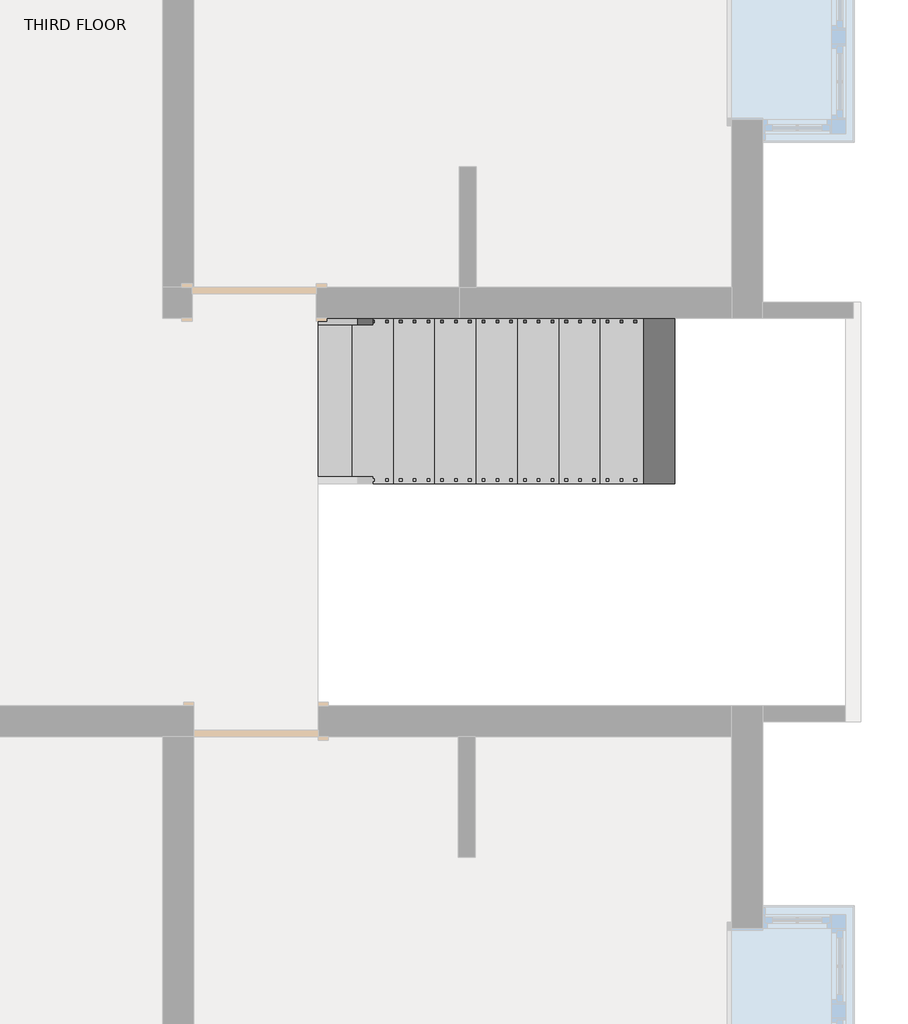
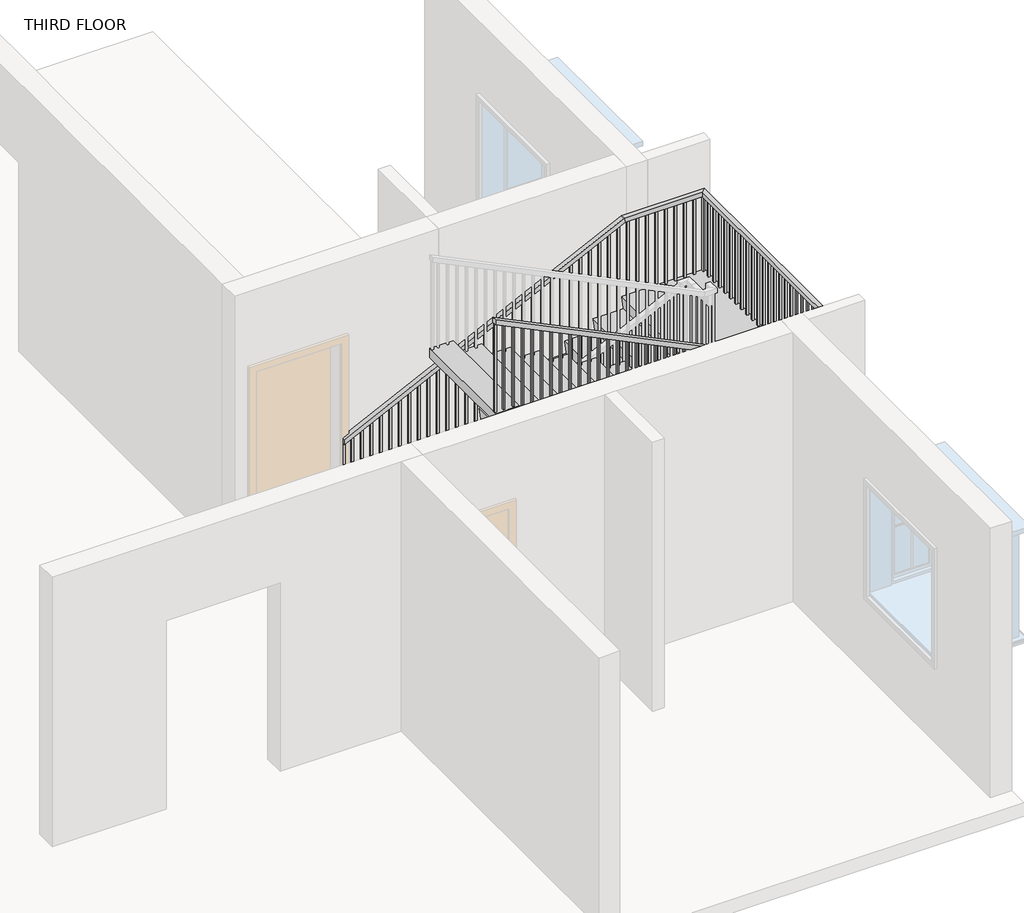
# One storey, part 3 of 4: 1 railing, 1 stair flight.
"""IFC4 building model written with IfcOpenShell, lengths in millimetres."""

from ifc_helpers import new_model, si_unit, frame, origin, place, context, project, spatial, polyline, outline, extrude, faceted_brep, element, save

model = new_model("IFC4")

# Units and contexts
model_context = context("Model", 3, world=origin())
ifc_project = project(units=[si_unit("LENGTHUNIT", "METRE", prefix="MILLI")], contexts=[model_context])

# Site, building, storey
site = spatial("IfcSite", under=ifc_project)
building = spatial("IfcBuilding", under=site)
storey = spatial("IfcBuildingStorey", under=building, Name="THIRD FLOOR", Elevation=9601.2)

# Railing
placement = place(None, origin())
element("IfcRailing", 1, ObjectType="Handrail - Rectangular", at=placement, inside=storey, context=model_context, shape_type="SolidModel", body=[
    faceted_brep([(3126.2584916, 220.733346, 10661.0727273), (3126.2584916, 220.733346, 10604.5956113), (3126.2584916, 169.933346, 10604.5956113), (3126.2584916, 169.933346, 10661.0727273), (6120.7829507, 220.733346, 12115.8), (6132.4691705, 220.733346, 12065.0), (6132.4691705, 169.933346, 12065.0), (6120.7829507, 169.933346, 12115.8), (7009.1350459, 220.733346, 12115.8), (7009.1350459, 220.733346, 12065.0), (6958.3350459, 169.933346, 12065.0), (6958.3350459, 169.933346, 12115.8), (7009.1350459, -2636.766654, 12115.8), (7009.1350459, -2636.766654, 12065.0), (6958.3350459, -2585.966654, 12065.0), (6958.3350459, -2585.966654, 12115.8), (6420.2353966, -2636.766654, 12115.8), (6408.5491768, -2636.766654, 12065.0), (6408.5491768, -2585.966654, 12065.0), (6420.2353966, -2585.966654, 12115.8), (3126.2584916, -2636.766654, 13716.0), (3126.2584916, -2585.966654, 13716.0), (3126.2584916, -2585.966654, 13659.522884), (3126.2584916, -2636.766654, 13659.522884)], [[[0, 1, 2, 3]], [[1, 0, 4, 5]], [[2, 1, 5, 6]], [[3, 2, 6, 7]], [[0, 3, 7, 4]], [[5, 4, 8, 9]], [[6, 5, 9, 10]], [[7, 6, 10, 11]], [[4, 7, 11, 8]], [[9, 8, 12, 13]], [[10, 9, 13, 14]], [[11, 10, 14, 15]], [[8, 11, 15, 12]], [[13, 12, 16, 17]], [[14, 13, 17, 18]], [[15, 14, 18, 19]], [[12, 15, 19, 16]], [[20, 21, 22, 23]], [[17, 16, 20, 23]], [[18, 17, 23, 22]], [[19, 18, 22, 21]], [[16, 19, 21, 20]]]),
    extrude(outline(polyline([(13616.4077556, 3215.0100459), (12656.1272727, 3215.0100459), (12656.1272727, 3234.0600459), (13607.1533465, 3234.0600459), (13616.4077556, 3215.0100459)])), frame((0.0, -2620.891654, 0.0), z_axis=(0.0, 1.0, 0.0), x_axis=(0.0, 0.0, 1.0)), (0.0, 0.0, 1.0), 19.05),
    extrude(outline(polyline([(13567.0509068, 3316.6100459), (12656.1272727, 3316.6100459), (12656.1272727, 3335.6600459), (13557.7964977, 3335.6600459), (13567.0509068, 3316.6100459)])), frame((0.0, -2620.891654, 0.0), z_axis=(0.0, 1.0, 0.0), x_axis=(0.0, 0.0, 1.0)), (0.0, 0.0, 1.0), 19.05),
    extrude(outline(polyline([(13517.694058, 3418.2100459), (12510.6545455, 3418.2100459), (12510.6545455, 3437.2600459), (13508.4396489, 3437.2600459), (13517.694058, 3418.2100459)])), frame((0.0, -2620.891654, 0.0), z_axis=(0.0, 1.0, 0.0), x_axis=(0.0, 0.0, 1.0)), (0.0, 0.0, 1.0), 19.05),
    extrude(outline(polyline([(13468.3372093, 3519.8100459), (12510.6545455, 3519.8100459), (12510.6545455, 3538.8600459), (13459.0828001, 3538.8600459), (13468.3372093, 3519.8100459)])), frame((0.0, -2620.891654, 0.0), z_axis=(0.0, 1.0, 0.0), x_axis=(0.0, 0.0, 1.0)), (0.0, 0.0, 1.0), 19.05),
    extrude(outline(polyline([(13418.9803605, 3621.4100459), (12510.6545455, 3621.4100459), (12510.6545455, 3640.4600459), (13409.7259513, 3640.4600459), (13418.9803605, 3621.4100459)])), frame((0.0, -2620.891654, 0.0), z_axis=(0.0, 1.0, 0.0), x_axis=(0.0, 0.0, 1.0)), (0.0, 0.0, 1.0), 19.05),
    extrude(outline(polyline([(13369.6235117, 3723.0100459), (12365.1818182, 3723.0100459), (12365.1818182, 3742.0600459), (13360.3691025, 3742.0600459), (13369.6235117, 3723.0100459)])), frame((0.0, -2620.891654, 0.0), z_axis=(0.0, 1.0, 0.0), x_axis=(0.0, 0.0, 1.0)), (0.0, 0.0, 1.0), 19.05),
    extrude(outline(polyline([(13320.2666629, 3824.6100459), (12365.1818182, 3824.6100459), (12365.1818182, 3843.6600459), (13311.0122538, 3843.6600459), (13320.2666629, 3824.6100459)])), frame((0.0, -2620.891654, 0.0), z_axis=(0.0, 1.0, 0.0), x_axis=(0.0, 0.0, 1.0)), (0.0, 0.0, 1.0), 19.05),
    extrude(outline(polyline([(13270.9098141, 3926.2100459), (12365.1818182, 3926.2100459), (12365.1818182, 3945.2600459), (13261.655405, 3945.2600459), (13270.9098141, 3926.2100459)])), frame((0.0, -2620.891654, 0.0), z_axis=(0.0, 1.0, 0.0), x_axis=(0.0, 0.0, 1.0)), (0.0, 0.0, 1.0), 19.05),
    extrude(outline(polyline([(13221.5529653, 4027.8100459), (12219.7090909, 4027.8100459), (12219.7090909, 4046.8600459), (13212.2985562, 4046.8600459), (13221.5529653, 4027.8100459)])), frame((0.0, -2620.891654, 0.0), z_axis=(0.0, 1.0, 0.0), x_axis=(0.0, 0.0, 1.0)), (0.0, 0.0, 1.0), 19.05),
    extrude(outline(polyline([(13172.1961165, 4129.4100459), (12219.7090909, 4129.4100459), (12219.7090909, 4148.4600459), (13162.9417074, 4148.4600459), (13172.1961165, 4129.4100459)])), frame((0.0, -2620.891654, 0.0), z_axis=(0.0, 1.0, 0.0), x_axis=(0.0, 0.0, 1.0)), (0.0, 0.0, 1.0), 19.05),
    extrude(outline(polyline([(13122.8392678, 4231.0100459), (12219.7090909, 4231.0100459), (12219.7090909, 4250.0600459), (13113.5848586, 4250.0600459), (13122.8392678, 4231.0100459)])), frame((0.0, -2620.891654, 0.0), z_axis=(0.0, 1.0, 0.0), x_axis=(0.0, 0.0, 1.0)), (0.0, 0.0, 1.0), 19.05),
    extrude(outline(polyline([(13073.482419, 4332.6100459), (12074.2363636, 4332.6100459), (12074.2363636, 4351.6600459), (13064.2280098, 4351.6600459), (13073.482419, 4332.6100459)])), frame((0.0, -2620.891654, 0.0), z_axis=(0.0, 1.0, 0.0), x_axis=(0.0, 0.0, 1.0)), (0.0, 0.0, 1.0), 19.05),
    extrude(outline(polyline([(13024.1255702, 4434.2100459), (12074.2363636, 4434.2100459), (12074.2363636, 4453.2600459), (13014.871161, 4453.2600459), (13024.1255702, 4434.2100459)])), frame((0.0, -2620.891654, 0.0), z_axis=(0.0, 1.0, 0.0), x_axis=(0.0, 0.0, 1.0)), (0.0, 0.0, 1.0), 19.05),
    extrude(outline(polyline([(12974.7687214, 4535.8100459), (12074.2363636, 4535.8100459), (12074.2363636, 4554.8600459), (12965.5143123, 4554.8600459), (12974.7687214, 4535.8100459)])), frame((0.0, -2620.891654, 0.0), z_axis=(0.0, 1.0, 0.0), x_axis=(0.0, 0.0, 1.0)), (0.0, 0.0, 1.0), 19.05),
    extrude(outline(polyline([(12925.4118726, 4637.4100459), (11928.7636364, 4637.4100459), (11928.7636364, 4656.4600459), (12916.1574635, 4656.4600459), (12925.4118726, 4637.4100459)])), frame((0.0, -2620.891654, 0.0), z_axis=(0.0, 1.0, 0.0), x_axis=(0.0, 0.0, 1.0)), (0.0, 0.0, 1.0), 19.05),
    extrude(outline(polyline([(12876.0550238, 4739.0100459), (11928.7636364, 4739.0100459), (11928.7636364, 4758.0600459), (12866.8006147, 4758.0600459), (12876.0550238, 4739.0100459)])), frame((0.0, -2620.891654, 0.0), z_axis=(0.0, 1.0, 0.0), x_axis=(0.0, 0.0, 1.0)), (0.0, 0.0, 1.0), 19.05),
    extrude(outline(polyline([(12826.6981751, 4840.6100459), (11928.7636364, 4840.6100459), (11928.7636364, 4859.6600459), (12817.4437659, 4859.6600459), (12826.6981751, 4840.6100459)])), frame((0.0, -2620.891654, 0.0), z_axis=(0.0, 1.0, 0.0), x_axis=(0.0, 0.0, 1.0)), (0.0, 0.0, 1.0), 19.05),
    extrude(outline(polyline([(12777.3413263, 4942.2100459), (11783.2909091, 4942.2100459), (11783.2909091, 4961.2600459), (12768.0869171, 4961.2600459), (12777.3413263, 4942.2100459)])), frame((0.0, -2620.891654, 0.0), z_axis=(0.0, 1.0, 0.0), x_axis=(0.0, 0.0, 1.0)), (0.0, 0.0, 1.0), 19.05),
    extrude(outline(polyline([(12727.9844775, 5043.8100459), (11783.2909091, 5043.8100459), (11783.2909091, 5062.8600459), (12718.7300683, 5062.8600459), (12727.9844775, 5043.8100459)])), frame((0.0, -2620.891654, 0.0), z_axis=(0.0, 1.0, 0.0), x_axis=(0.0, 0.0, 1.0)), (0.0, 0.0, 1.0), 19.05),
    extrude(outline(polyline([(12678.6276287, 5145.4100459), (11783.2909091, 5145.4100459), (11783.2909091, 5164.4600459), (12669.3732196, 5164.4600459), (12678.6276287, 5145.4100459)])), frame((0.0, -2620.891654, 0.0), z_axis=(0.0, 1.0, 0.0), x_axis=(0.0, 0.0, 1.0)), (0.0, 0.0, 1.0), 19.05),
    extrude(outline(polyline([(12629.2707799, 5247.0100459), (11637.8181818, 5247.0100459), (11637.8181818, 5266.0600459), (12620.0163708, 5266.0600459), (12629.2707799, 5247.0100459)])), frame((0.0, -2620.891654, 0.0), z_axis=(0.0, 1.0, 0.0), x_axis=(0.0, 0.0, 1.0)), (0.0, 0.0, 1.0), 19.05),
    extrude(outline(polyline([(12579.9139311, 5348.6100459), (11637.8181818, 5348.6100459), (11637.8181818, 5367.6600459), (12570.659522, 5367.6600459), (12579.9139311, 5348.6100459)])), frame((0.0, -2620.891654, 0.0), z_axis=(0.0, 1.0, 0.0), x_axis=(0.0, 0.0, 1.0)), (0.0, 0.0, 1.0), 19.05),
    extrude(outline(polyline([(12530.5570823, 5450.2100459), (11637.8181818, 5450.2100459), (11637.8181818, 5469.2600459), (12521.3026732, 5469.2600459), (12530.5570823, 5450.2100459)])), frame((0.0, -2620.891654, 0.0), z_axis=(0.0, 1.0, 0.0), x_axis=(0.0, 0.0, 1.0)), (0.0, 0.0, 1.0), 19.05),
    extrude(outline(polyline([(12481.2002336, 5551.8100459), (11492.3454545, 5551.8100459), (11492.3454545, 5570.8600459), (12471.9458244, 5570.8600459), (12481.2002336, 5551.8100459)])), frame((0.0, -2620.891654, 0.0), z_axis=(0.0, 1.0, 0.0), x_axis=(0.0, 0.0, 1.0)), (0.0, 0.0, 1.0), 19.05),
    extrude(outline(polyline([(12431.8433848, 5653.4100459), (11492.3454545, 5653.4100459), (11492.3454545, 5672.4600459), (12422.5889756, 5672.4600459), (12431.8433848, 5653.4100459)])), frame((0.0, -2620.891654, 0.0), z_axis=(0.0, 1.0, 0.0), x_axis=(0.0, 0.0, 1.0)), (0.0, 0.0, 1.0), 19.05),
    extrude(outline(polyline([(12382.486536, 5755.0100459), (11492.3454545, 5755.0100459), (11492.3454545, 5774.0600459), (12373.2321268, 5774.0600459), (12382.486536, 5755.0100459)])), frame((0.0, -2620.891654, 0.0), z_axis=(0.0, 1.0, 0.0), x_axis=(0.0, 0.0, 1.0)), (0.0, 0.0, 1.0), 19.05),
    extrude(outline(polyline([(12333.1296872, 5856.6100459), (11346.8727273, 5856.6100459), (11346.8727273, 5875.6600459), (12323.8752781, 5875.6600459), (12333.1296872, 5856.6100459)])), frame((0.0, -2620.891654, 0.0), z_axis=(0.0, 1.0, 0.0), x_axis=(0.0, 0.0, 1.0)), (0.0, 0.0, 1.0), 19.05),
    extrude(outline(polyline([(12283.7728384, 5958.2100459), (11346.8727273, 5958.2100459), (11346.8727273, 5977.2600459), (12274.5184293, 5977.2600459), (12283.7728384, 5958.2100459)])), frame((0.0, -2620.891654, 0.0), z_axis=(0.0, 1.0, 0.0), x_axis=(0.0, 0.0, 1.0)), (0.0, 0.0, 1.0), 19.05),
    extrude(outline(polyline([(12234.4159896, 6059.8100459), (11346.8727273, 6059.8100459), (11346.8727273, 6078.8600459), (12225.1615805, 6078.8600459), (12234.4159896, 6059.8100459)])), frame((0.0, -2620.891654, 0.0), z_axis=(0.0, 1.0, 0.0), x_axis=(0.0, 0.0, 1.0)), (0.0, 0.0, 1.0), 19.05),
    extrude(outline(polyline([(12185.0591409, 6161.4100459), (11201.4, 6161.4100459), (11201.4, 6180.4600459), (12175.8047317, 6180.4600459), (12185.0591409, 6161.4100459)])), frame((0.0, -2620.891654, 0.0), z_axis=(0.0, 1.0, 0.0), x_axis=(0.0, 0.0, 1.0)), (0.0, 0.0, 1.0), 19.05),
    extrude(outline(polyline([(12135.7022921, 6263.0100459), (11201.4, 6263.0100459), (11201.4, 6282.0600459), (12126.4478829, 6282.0600459), (12135.7022921, 6263.0100459)])), frame((0.0, -2620.891654, 0.0), z_axis=(0.0, 1.0, 0.0), x_axis=(0.0, 0.0, 1.0)), (0.0, 0.0, 1.0), 19.05),
    extrude(outline(polyline([(12086.3454433, 6364.6100459), (11201.4, 6364.6100459), (11201.4, 6383.6600459), (12077.0910341, 6383.6600459), (12086.3454433, 6364.6100459)])), frame((0.0, -2620.891654, 0.0), z_axis=(0.0, 1.0, 0.0), x_axis=(0.0, 0.0, 1.0)), (0.0, 0.0, 1.0), 19.05),
    extrude(outline(polyline([(6485.2600459, -2620.891654), (6466.2100459, -2620.891654), (6466.2100459, -2601.841654), (6485.2600459, -2601.841654), (6485.2600459, -2620.891654)])), frame((0.0, 0.0, 11201.4), z_axis=(0.0, 0.0, 1.0), x_axis=(1.0, 0.0, 0.0)), (0.0, 0.0, 1.0), 863.6),
    extrude(outline(polyline([(6586.8600459, -2620.891654), (6567.8100459, -2620.891654), (6567.8100459, -2601.841654), (6586.8600459, -2601.841654), (6586.8600459, -2620.891654)])), frame((0.0, 0.0, 11201.4), z_axis=(0.0, 0.0, 1.0), x_axis=(1.0, 0.0, 0.0)), (0.0, 0.0, 1.0), 863.6),
    extrude(outline(polyline([(6688.4600459, -2620.891654), (6669.4100459, -2620.891654), (6669.4100459, -2601.841654), (6688.4600459, -2601.841654), (6688.4600459, -2620.891654)])), frame((0.0, 0.0, 11201.4), z_axis=(0.0, 0.0, 1.0), x_axis=(1.0, 0.0, 0.0)), (0.0, 0.0, 1.0), 863.6),
    extrude(outline(polyline([(6790.0600459, -2620.891654), (6771.0100459, -2620.891654), (6771.0100459, -2601.841654), (6790.0600459, -2601.841654), (6790.0600459, -2620.891654)])), frame((0.0, 0.0, 11201.4), z_axis=(0.0, 0.0, 1.0), x_axis=(1.0, 0.0, 0.0)), (0.0, 0.0, 1.0), 863.6),
    extrude(outline(polyline([(6891.6600459, -2620.891654), (6872.6100459, -2620.891654), (6872.6100459, -2601.841654), (6891.6600459, -2601.841654), (6891.6600459, -2620.891654)])), frame((0.0, 0.0, 11201.4), z_axis=(0.0, 0.0, 1.0), x_axis=(1.0, 0.0, 0.0)), (0.0, 0.0, 1.0), 863.6),
    extrude(outline(polyline([(6993.2600459, -2538.341654), (6993.2600459, -2557.391654), (6974.2100459, -2557.391654), (6974.2100459, -2538.341654), (6993.2600459, -2538.341654)])), frame((0.0, 0.0, 11201.4), z_axis=(0.0, 0.0, 1.0), x_axis=(1.0, 0.0, 0.0)), (0.0, 0.0, 1.0), 863.6),
    extrude(outline(polyline([(6993.2600459, -2436.741654), (6993.2600459, -2455.791654), (6974.2100459, -2455.791654), (6974.2100459, -2436.741654), (6993.2600459, -2436.741654)])), frame((0.0, 0.0, 11201.4), z_axis=(0.0, 0.0, 1.0), x_axis=(1.0, 0.0, 0.0)), (0.0, 0.0, 1.0), 863.6),
    extrude(outline(polyline([(6993.2600459, -2335.141654), (6993.2600459, -2354.191654), (6974.2100459, -2354.191654), (6974.2100459, -2335.141654), (6993.2600459, -2335.141654)])), frame((0.0, 0.0, 11201.4), z_axis=(0.0, 0.0, 1.0), x_axis=(1.0, 0.0, 0.0)), (0.0, 0.0, 1.0), 863.6),
    extrude(outline(polyline([(6993.2600459, -2233.541654), (6993.2600459, -2252.591654), (6974.2100459, -2252.591654), (6974.2100459, -2233.541654), (6993.2600459, -2233.541654)])), frame((0.0, 0.0, 11201.4), z_axis=(0.0, 0.0, 1.0), x_axis=(1.0, 0.0, 0.0)), (0.0, 0.0, 1.0), 863.6),
    extrude(outline(polyline([(6993.2600459, -2131.941654), (6993.2600459, -2150.991654), (6974.2100459, -2150.991654), (6974.2100459, -2131.941654), (6993.2600459, -2131.941654)])), frame((0.0, 0.0, 11201.4), z_axis=(0.0, 0.0, 1.0), x_axis=(1.0, 0.0, 0.0)), (0.0, 0.0, 1.0), 863.6),
    extrude(outline(polyline([(6993.2600459, -2030.341654), (6993.2600459, -2049.391654), (6974.2100459, -2049.391654), (6974.2100459, -2030.341654), (6993.2600459, -2030.341654)])), frame((0.0, 0.0, 11201.4), z_axis=(0.0, 0.0, 1.0), x_axis=(1.0, 0.0, 0.0)), (0.0, 0.0, 1.0), 863.6),
    extrude(outline(polyline([(6993.2600459, -1928.741654), (6993.2600459, -1947.791654), (6974.2100459, -1947.791654), (6974.2100459, -1928.741654), (6993.2600459, -1928.741654)])), frame((0.0, 0.0, 11201.4), z_axis=(0.0, 0.0, 1.0), x_axis=(1.0, 0.0, 0.0)), (0.0, 0.0, 1.0), 863.6),
    extrude(outline(polyline([(6993.2600459, -1827.141654), (6993.2600459, -1846.191654), (6974.2100459, -1846.191654), (6974.2100459, -1827.141654), (6993.2600459, -1827.141654)])), frame((0.0, 0.0, 11201.4), z_axis=(0.0, 0.0, 1.0), x_axis=(1.0, 0.0, 0.0)), (0.0, 0.0, 1.0), 863.6),
    extrude(outline(polyline([(6993.2600459, -1725.541654), (6993.2600459, -1744.591654), (6974.2100459, -1744.591654), (6974.2100459, -1725.541654), (6993.2600459, -1725.541654)])), frame((0.0, 0.0, 11201.4), z_axis=(0.0, 0.0, 1.0), x_axis=(1.0, 0.0, 0.0)), (0.0, 0.0, 1.0), 863.6),
    extrude(outline(polyline([(6993.2600459, -1623.941654), (6993.2600459, -1642.991654), (6974.2100459, -1642.991654), (6974.2100459, -1623.941654), (6993.2600459, -1623.941654)])), frame((0.0, 0.0, 11201.4), z_axis=(0.0, 0.0, 1.0), x_axis=(1.0, 0.0, 0.0)), (0.0, 0.0, 1.0), 863.6),
    extrude(outline(polyline([(6993.2600459, -1522.341654), (6993.2600459, -1541.391654), (6974.2100459, -1541.391654), (6974.2100459, -1522.341654), (6993.2600459, -1522.341654)])), frame((0.0, 0.0, 11201.4), z_axis=(0.0, 0.0, 1.0), x_axis=(1.0, 0.0, 0.0)), (0.0, 0.0, 1.0), 863.6),
    extrude(outline(polyline([(6993.2600459, -1420.741654), (6993.2600459, -1439.791654), (6974.2100459, -1439.791654), (6974.2100459, -1420.741654), (6993.2600459, -1420.741654)])), frame((0.0, 0.0, 11201.4), z_axis=(0.0, 0.0, 1.0), x_axis=(1.0, 0.0, 0.0)), (0.0, 0.0, 1.0), 863.6),
    extrude(outline(polyline([(6993.2600459, -1319.141654), (6993.2600459, -1338.191654), (6974.2100459, -1338.191654), (6974.2100459, -1319.141654), (6993.2600459, -1319.141654)])), frame((0.0, 0.0, 11201.4), z_axis=(0.0, 0.0, 1.0), x_axis=(1.0, 0.0, 0.0)), (0.0, 0.0, 1.0), 863.6),
    extrude(outline(polyline([(6993.2600459, -1217.541654), (6993.2600459, -1236.591654), (6974.2100459, -1236.591654), (6974.2100459, -1217.541654), (6993.2600459, -1217.541654)])), frame((0.0, 0.0, 11201.4), z_axis=(0.0, 0.0, 1.0), x_axis=(1.0, 0.0, 0.0)), (0.0, 0.0, 1.0), 863.6),
    extrude(outline(polyline([(6993.2600459, -1115.941654), (6993.2600459, -1134.991654), (6974.2100459, -1134.991654), (6974.2100459, -1115.941654), (6993.2600459, -1115.941654)])), frame((0.0, 0.0, 11201.4), z_axis=(0.0, 0.0, 1.0), x_axis=(1.0, 0.0, 0.0)), (0.0, 0.0, 1.0), 863.6),
    extrude(outline(polyline([(6993.2600459, -1014.341654), (6993.2600459, -1033.391654), (6974.2100459, -1033.391654), (6974.2100459, -1014.341654), (6993.2600459, -1014.341654)])), frame((0.0, 0.0, 11201.4), z_axis=(0.0, 0.0, 1.0), x_axis=(1.0, 0.0, 0.0)), (0.0, 0.0, 1.0), 863.6),
    extrude(outline(polyline([(6993.2600459, -912.741654), (6993.2600459, -931.791654), (6974.2100459, -931.791654), (6974.2100459, -912.741654), (6993.2600459, -912.741654)])), frame((0.0, 0.0, 11201.4), z_axis=(0.0, 0.0, 1.0), x_axis=(1.0, 0.0, 0.0)), (0.0, 0.0, 1.0), 863.6),
    extrude(outline(polyline([(6993.2600459, -811.141654), (6993.2600459, -830.191654), (6974.2100459, -830.191654), (6974.2100459, -811.141654), (6993.2600459, -811.141654)])), frame((0.0, 0.0, 11201.4), z_axis=(0.0, 0.0, 1.0), x_axis=(1.0, 0.0, 0.0)), (0.0, 0.0, 1.0), 863.6),
    extrude(outline(polyline([(6993.2600459, -709.541654), (6993.2600459, -728.591654), (6974.2100459, -728.591654), (6974.2100459, -709.541654), (6993.2600459, -709.541654)])), frame((0.0, 0.0, 11201.4), z_axis=(0.0, 0.0, 1.0), x_axis=(1.0, 0.0, 0.0)), (0.0, 0.0, 1.0), 863.6),
    extrude(outline(polyline([(6993.2600459, -607.941654), (6993.2600459, -626.991654), (6974.2100459, -626.991654), (6974.2100459, -607.941654), (6993.2600459, -607.941654)])), frame((0.0, 0.0, 11201.4), z_axis=(0.0, 0.0, 1.0), x_axis=(1.0, 0.0, 0.0)), (0.0, 0.0, 1.0), 863.6),
    extrude(outline(polyline([(6993.2600459, -506.341654), (6993.2600459, -525.391654), (6974.2100459, -525.391654), (6974.2100459, -506.341654), (6993.2600459, -506.341654)])), frame((0.0, 0.0, 11201.4), z_axis=(0.0, 0.0, 1.0), x_axis=(1.0, 0.0, 0.0)), (0.0, 0.0, 1.0), 863.6),
    extrude(outline(polyline([(6993.2600459, -404.741654), (6993.2600459, -423.791654), (6974.2100459, -423.791654), (6974.2100459, -404.741654), (6993.2600459, -404.741654)])), frame((0.0, 0.0, 11201.4), z_axis=(0.0, 0.0, 1.0), x_axis=(1.0, 0.0, 0.0)), (0.0, 0.0, 1.0), 863.6),
    extrude(outline(polyline([(6993.2600459, -303.141654), (6993.2600459, -322.191654), (6974.2100459, -322.191654), (6974.2100459, -303.141654), (6993.2600459, -303.141654)])), frame((0.0, 0.0, 11201.4), z_axis=(0.0, 0.0, 1.0), x_axis=(1.0, 0.0, 0.0)), (0.0, 0.0, 1.0), 863.6),
    extrude(outline(polyline([(6993.2600459, -201.541654), (6993.2600459, -220.591654), (6974.2100459, -220.591654), (6974.2100459, -201.541654), (6993.2600459, -201.541654)])), frame((0.0, 0.0, 11201.4), z_axis=(0.0, 0.0, 1.0), x_axis=(1.0, 0.0, 0.0)), (0.0, 0.0, 1.0), 863.6),
    extrude(outline(polyline([(6993.2600459, -99.941654), (6993.2600459, -118.991654), (6974.2100459, -118.991654), (6974.2100459, -99.941654), (6993.2600459, -99.941654)])), frame((0.0, 0.0, 11201.4), z_axis=(0.0, 0.0, 1.0), x_axis=(1.0, 0.0, 0.0)), (0.0, 0.0, 1.0), 863.6),
    extrude(outline(polyline([(6993.2600459, 1.658346), (6993.2600459, -17.391654), (6974.2100459, -17.391654), (6974.2100459, 1.658346), (6993.2600459, 1.658346)])), frame((0.0, 0.0, 11201.4), z_axis=(0.0, 0.0, 1.0), x_axis=(1.0, 0.0, 0.0)), (0.0, 0.0, 1.0), 863.6),
    extrude(outline(polyline([(6993.2600459, 103.258346), (6993.2600459, 84.208346), (6974.2100459, 84.208346), (6974.2100459, 103.258346), (6993.2600459, 103.258346)])), frame((0.0, 0.0, 11201.4), z_axis=(0.0, 0.0, 1.0), x_axis=(1.0, 0.0, 0.0)), (0.0, 0.0, 1.0), 863.6),
    extrude(outline(polyline([(6875.9334916, 204.858346), (6894.9834916, 204.858346), (6894.9834916, 185.808346), (6875.9334916, 185.808346), (6875.9334916, 204.858346)])), frame((0.0, 0.0, 11201.4), z_axis=(0.0, 0.0, 1.0), x_axis=(1.0, 0.0, 0.0)), (0.0, 0.0, 1.0), 863.6),
    extrude(outline(polyline([(6774.3334916, 204.858346), (6793.3834916, 204.858346), (6793.3834916, 185.808346), (6774.3334916, 185.808346), (6774.3334916, 204.858346)])), frame((0.0, 0.0, 11201.4), z_axis=(0.0, 0.0, 1.0), x_axis=(1.0, 0.0, 0.0)), (0.0, 0.0, 1.0), 863.6),
    extrude(outline(polyline([(6672.7334916, 204.858346), (6691.7834916, 204.858346), (6691.7834916, 185.808346), (6672.7334916, 185.808346), (6672.7334916, 204.858346)])), frame((0.0, 0.0, 11201.4), z_axis=(0.0, 0.0, 1.0), x_axis=(1.0, 0.0, 0.0)), (0.0, 0.0, 1.0), 863.6),
    extrude(outline(polyline([(6571.1334916, 204.858346), (6590.1834916, 204.858346), (6590.1834916, 185.808346), (6571.1334916, 185.808346), (6571.1334916, 204.858346)])), frame((0.0, 0.0, 11201.4), z_axis=(0.0, 0.0, 1.0), x_axis=(1.0, 0.0, 0.0)), (0.0, 0.0, 1.0), 863.6),
    extrude(outline(polyline([(6469.5334916, 204.858346), (6488.5834916, 204.858346), (6488.5834916, 185.808346), (6469.5334916, 185.808346), (6469.5334916, 204.858346)])), frame((0.0, 0.0, 11201.4), z_axis=(0.0, 0.0, 1.0), x_axis=(1.0, 0.0, 0.0)), (0.0, 0.0, 1.0), 863.6),
    extrude(outline(polyline([(6367.9334916, 204.858346), (6386.9834916, 204.858346), (6386.9834916, 185.808346), (6367.9334916, 185.808346), (6367.9334916, 204.858346)])), frame((0.0, 0.0, 11201.4), z_axis=(0.0, 0.0, 1.0), x_axis=(1.0, 0.0, 0.0)), (0.0, 0.0, 1.0), 863.6),
    extrude(outline(polyline([(6266.3334916, 204.858346), (6285.3834916, 204.858346), (6285.3834916, 185.808346), (6266.3334916, 185.808346), (6266.3334916, 204.858346)])), frame((0.0, 0.0, 11201.4), z_axis=(0.0, 0.0, 1.0), x_axis=(1.0, 0.0, 0.0)), (0.0, 0.0, 1.0), 863.6),
    extrude(outline(polyline([(6164.7334916, 204.858346), (6183.7834916, 204.858346), (6183.7834916, 185.808346), (6164.7334916, 185.808346), (6164.7334916, 204.858346)])), frame((0.0, 0.0, 11201.4), z_axis=(0.0, 0.0, 1.0), x_axis=(1.0, 0.0, 0.0)), (0.0, 0.0, 1.0), 863.6),
    extrude(outline(polyline([(12031.3170215, 6063.1334916), (11055.9272727, 6063.1334916), (11055.9272727, 6082.1834916), (12040.5714306, 6082.1834916), (12031.3170215, 6063.1334916)])), frame((0.0, 185.808346, 0.0), z_axis=(0.0, 1.0, 0.0), x_axis=(0.0, 0.0, 1.0)), (0.0, 0.0, 1.0), 19.05),
    extrude(outline(polyline([(11981.9601727, 5961.5334916), (11055.9272727, 5961.5334916), (11055.9272727, 5980.5834916), (11991.2145818, 5980.5834916), (11981.9601727, 5961.5334916)])), frame((0.0, 185.808346, 0.0), z_axis=(0.0, 1.0, 0.0), x_axis=(0.0, 0.0, 1.0)), (0.0, 0.0, 1.0), 19.05),
    extrude(outline(polyline([(11932.6033239, 5859.9334916), (11055.9272727, 5859.9334916), (11055.9272727, 5878.9834916), (11941.857733, 5878.9834916), (11932.6033239, 5859.9334916)])), frame((0.0, 185.808346, 0.0), z_axis=(0.0, 1.0, 0.0), x_axis=(0.0, 0.0, 1.0)), (0.0, 0.0, 1.0), 19.05),
    extrude(outline(polyline([(11883.2464751, 5758.3334916), (10910.4545455, 5758.3334916), (10910.4545455, 5777.3834916), (11892.5008843, 5777.3834916), (11883.2464751, 5758.3334916)])), frame((0.0, 185.808346, 0.0), z_axis=(0.0, 1.0, 0.0), x_axis=(0.0, 0.0, 1.0)), (0.0, 0.0, 1.0), 19.05),
    extrude(outline(polyline([(11833.8896263, 5656.7334916), (10910.4545455, 5656.7334916), (10910.4545455, 5675.7834916), (11843.1440355, 5675.7834916), (11833.8896263, 5656.7334916)])), frame((0.0, 185.808346, 0.0), z_axis=(0.0, 1.0, 0.0), x_axis=(0.0, 0.0, 1.0)), (0.0, 0.0, 1.0), 19.05),
    extrude(outline(polyline([(11784.5327775, 5555.1334916), (10910.4545455, 5555.1334916), (10910.4545455, 5574.1834916), (11793.7871867, 5574.1834916), (11784.5327775, 5555.1334916)])), frame((0.0, 185.808346, 0.0), z_axis=(0.0, 1.0, 0.0), x_axis=(0.0, 0.0, 1.0)), (0.0, 0.0, 1.0), 19.05),
    extrude(outline(polyline([(11735.1759288, 5453.5334916), (10764.9818182, 5453.5334916), (10764.9818182, 5472.5834916), (11744.4303379, 5472.5834916), (11735.1759288, 5453.5334916)])), frame((0.0, 185.808346, 0.0), z_axis=(0.0, 1.0, 0.0), x_axis=(0.0, 0.0, 1.0)), (0.0, 0.0, 1.0), 19.05),
    extrude(outline(polyline([(11685.81908, 5351.9334916), (10764.9818182, 5351.9334916), (10764.9818182, 5370.9834916), (11695.0734891, 5370.9834916), (11685.81908, 5351.9334916)])), frame((0.0, 185.808346, 0.0), z_axis=(0.0, 1.0, 0.0), x_axis=(0.0, 0.0, 1.0)), (0.0, 0.0, 1.0), 19.05),
    extrude(outline(polyline([(11636.4622312, 5250.3334916), (10764.9818182, 5250.3334916), (10764.9818182, 5269.3834916), (11645.7166403, 5269.3834916), (11636.4622312, 5250.3334916)])), frame((0.0, 185.808346, 0.0), z_axis=(0.0, 1.0, 0.0), x_axis=(0.0, 0.0, 1.0)), (0.0, 0.0, 1.0), 19.05),
    extrude(outline(polyline([(11587.1053824, 5148.7334916), (10619.5090909, 5148.7334916), (10619.5090909, 5167.7834916), (11596.3597915, 5167.7834916), (11587.1053824, 5148.7334916)])), frame((0.0, 185.808346, 0.0), z_axis=(0.0, 1.0, 0.0), x_axis=(0.0, 0.0, 1.0)), (0.0, 0.0, 1.0), 19.05),
    extrude(outline(polyline([(11537.7485336, 5047.1334916), (10619.5090909, 5047.1334916), (10619.5090909, 5066.1834916), (11547.0029428, 5066.1834916), (11537.7485336, 5047.1334916)])), frame((0.0, 185.808346, 0.0), z_axis=(0.0, 1.0, 0.0), x_axis=(0.0, 0.0, 1.0)), (0.0, 0.0, 1.0), 19.05),
    extrude(outline(polyline([(11488.3916848, 4945.5334916), (10619.5090909, 4945.5334916), (10619.5090909, 4964.5834916), (11497.646094, 4964.5834916), (11488.3916848, 4945.5334916)])), frame((0.0, 185.808346, 0.0), z_axis=(0.0, 1.0, 0.0), x_axis=(0.0, 0.0, 1.0)), (0.0, 0.0, 1.0), 19.05),
    extrude(outline(polyline([(11439.034836, 4843.9334916), (10474.0363636, 4843.9334916), (10474.0363636, 4862.9834916), (11448.2892452, 4862.9834916), (11439.034836, 4843.9334916)])), frame((0.0, 185.808346, 0.0), z_axis=(0.0, 1.0, 0.0), x_axis=(0.0, 0.0, 1.0)), (0.0, 0.0, 1.0), 19.05),
    extrude(outline(polyline([(11389.6779873, 4742.3334916), (10474.0363636, 4742.3334916), (10474.0363636, 4761.3834916), (11398.9323964, 4761.3834916), (11389.6779873, 4742.3334916)])), frame((0.0, 185.808346, 0.0), z_axis=(0.0, 1.0, 0.0), x_axis=(0.0, 0.0, 1.0)), (0.0, 0.0, 1.0), 19.05),
    extrude(outline(polyline([(11340.3211385, 4640.7334916), (10474.0363636, 4640.7334916), (10474.0363636, 4659.7834916), (11349.5755476, 4659.7834916), (11340.3211385, 4640.7334916)])), frame((0.0, 185.808346, 0.0), z_axis=(0.0, 1.0, 0.0), x_axis=(0.0, 0.0, 1.0)), (0.0, 0.0, 1.0), 19.05),
    extrude(outline(polyline([(11290.9642897, 4539.1334916), (10328.5636364, 4539.1334916), (10328.5636364, 4558.1834916), (11300.2186988, 4558.1834916), (11290.9642897, 4539.1334916)])), frame((0.0, 185.808346, 0.0), z_axis=(0.0, 1.0, 0.0), x_axis=(0.0, 0.0, 1.0)), (0.0, 0.0, 1.0), 19.05),
    extrude(outline(polyline([(11241.6074409, 4437.5334916), (10328.5636364, 4437.5334916), (10328.5636364, 4456.5834916), (11250.8618501, 4456.5834916), (11241.6074409, 4437.5334916)])), frame((0.0, 185.808346, 0.0), z_axis=(0.0, 1.0, 0.0), x_axis=(0.0, 0.0, 1.0)), (0.0, 0.0, 1.0), 19.05),
    extrude(outline(polyline([(11192.2505921, 4335.9334916), (10328.5636364, 4335.9334916), (10328.5636364, 4354.9834916), (11201.5050013, 4354.9834916), (11192.2505921, 4335.9334916)])), frame((0.0, 185.808346, 0.0), z_axis=(0.0, 1.0, 0.0), x_axis=(0.0, 0.0, 1.0)), (0.0, 0.0, 1.0), 19.05),
    extrude(outline(polyline([(11142.8937433, 4234.3334916), (10183.0909091, 4234.3334916), (10183.0909091, 4253.3834916), (11152.1481525, 4253.3834916), (11142.8937433, 4234.3334916)])), frame((0.0, 185.808346, 0.0), z_axis=(0.0, 1.0, 0.0), x_axis=(0.0, 0.0, 1.0)), (0.0, 0.0, 1.0), 19.05),
    extrude(outline(polyline([(11093.5368946, 4132.7334916), (10183.0909091, 4132.7334916), (10183.0909091, 4151.7834916), (11102.7913037, 4151.7834916), (11093.5368946, 4132.7334916)])), frame((0.0, 185.808346, 0.0), z_axis=(0.0, 1.0, 0.0), x_axis=(0.0, 0.0, 1.0)), (0.0, 0.0, 1.0), 19.05),
    extrude(outline(polyline([(11044.1800458, 4031.1334916), (10183.0909091, 4031.1334916), (10183.0909091, 4050.1834916), (11053.4344549, 4050.1834916), (11044.1800458, 4031.1334916)])), frame((0.0, 185.808346, 0.0), z_axis=(0.0, 1.0, 0.0), x_axis=(0.0, 0.0, 1.0)), (0.0, 0.0, 1.0), 19.05),
    extrude(outline(polyline([(10994.823197, 3929.5334916), (10037.6181818, 3929.5334916), (10037.6181818, 3948.5834916), (11004.0776061, 3948.5834916), (10994.823197, 3929.5334916)])), frame((0.0, 185.808346, 0.0), z_axis=(0.0, 1.0, 0.0), x_axis=(0.0, 0.0, 1.0)), (0.0, 0.0, 1.0), 19.05),
    extrude(outline(polyline([(10945.4663482, 3827.9334916), (10037.6181818, 3827.9334916), (10037.6181818, 3846.9834916), (10954.7207573, 3846.9834916), (10945.4663482, 3827.9334916)])), frame((0.0, 185.808346, 0.0), z_axis=(0.0, 1.0, 0.0), x_axis=(0.0, 0.0, 1.0)), (0.0, 0.0, 1.0), 19.05),
    extrude(outline(polyline([(10896.1094994, 3726.3334916), (10037.6181818, 3726.3334916), (10037.6181818, 3745.3834916), (10905.3639086, 3745.3834916), (10896.1094994, 3726.3334916)])), frame((0.0, 185.808346, 0.0), z_axis=(0.0, 1.0, 0.0), x_axis=(0.0, 0.0, 1.0)), (0.0, 0.0, 1.0), 19.05),
    extrude(outline(polyline([(10846.7526506, 3624.7334916), (9892.1454545, 3624.7334916), (9892.1454545, 3643.7834916), (10856.0070598, 3643.7834916), (10846.7526506, 3624.7334916)])), frame((0.0, 185.808346, 0.0), z_axis=(0.0, 1.0, 0.0), x_axis=(0.0, 0.0, 1.0)), (0.0, 0.0, 1.0), 19.05),
    extrude(outline(polyline([(10797.3958018, 3523.1334916), (9892.1454545, 3523.1334916), (9892.1454545, 3542.1834916), (10806.650211, 3542.1834916), (10797.3958018, 3523.1334916)])), frame((0.0, 185.808346, 0.0), z_axis=(0.0, 1.0, 0.0), x_axis=(0.0, 0.0, 1.0)), (0.0, 0.0, 1.0), 19.05),
    extrude(outline(polyline([(10748.0389531, 3421.5334916), (9892.1454545, 3421.5334916), (9892.1454545, 3440.5834916), (10757.2933622, 3440.5834916), (10748.0389531, 3421.5334916)])), frame((0.0, 185.808346, 0.0), z_axis=(0.0, 1.0, 0.0), x_axis=(0.0, 0.0, 1.0)), (0.0, 0.0, 1.0), 19.05),
    extrude(outline(polyline([(10698.6821043, 3319.9334916), (9746.6727273, 3319.9334916), (9746.6727273, 3338.9834916), (10707.9365134, 3338.9834916), (10698.6821043, 3319.9334916)])), frame((0.0, 185.808346, 0.0), z_axis=(0.0, 1.0, 0.0), x_axis=(0.0, 0.0, 1.0)), (0.0, 0.0, 1.0), 19.05),
    extrude(outline(polyline([(10649.3252555, 3218.3334916), (9746.6727273, 3218.3334916), (9746.6727273, 3237.3834916), (10658.5796646, 3237.3834916), (10649.3252555, 3218.3334916)])), frame((0.0, 185.808346, 0.0), z_axis=(0.0, 1.0, 0.0), x_axis=(0.0, 0.0, 1.0)), (0.0, 0.0, 1.0), 19.05),
    extrude(outline(polyline([(6993.2600459, -2601.841654), (6993.2600459, -2620.891654), (6974.2100459, -2620.891654), (6974.2100459, -2601.841654), (6993.2600459, -2601.841654)])), frame((0.0, 0.0, 11201.4), z_axis=(0.0, 0.0, 1.0), x_axis=(1.0, 0.0, 0.0)), (0.0, 0.0, 1.0), 863.6),
    extrude(outline(polyline([(6974.2100459, 204.858346), (6993.2600459, 204.858346), (6993.2600459, 185.808346), (6974.2100459, 185.808346), (6974.2100459, 204.858346)])), frame((0.0, 0.0, 11201.4), z_axis=(0.0, 0.0, 1.0), x_axis=(1.0, 0.0, 0.0)), (0.0, 0.0, 1.0), 863.6),
    extrude(outline(polyline([(13659.522884, 3126.2584916), (12656.1272727, 3126.2584916), (12656.1272727, 3145.3084916), (13650.2684749, 3145.3084916), (13659.522884, 3126.2584916)])), frame((0.0, -2620.891654, 0.0), z_axis=(0.0, 1.0, 0.0), x_axis=(0.0, 0.0, 1.0)), (0.0, 0.0, 1.0), 19.05),
    extrude(outline(polyline([(10604.5956113, 3126.2584916), (9746.6727273, 3126.2584916), (9746.6727273, 3145.3084916), (10613.8500204, 3145.3084916), (10604.5956113, 3126.2584916)])), frame((0.0, 185.808346, 0.0), z_axis=(0.0, 1.0, 0.0), x_axis=(0.0, 0.0, 1.0)), (0.0, 0.0, 1.0), 19.05),
])

# Stair flight
element("IfcStairFlight", 2, ObjectType="3/4\" Nosing", at=placement, inside=storey, context=model_context, shape_type="Brep", body=[
    faceted_brep([(3126.2584916, 220.733346, 9746.6727273), (3126.2584916, -998.466654, 9746.6727273), (3396.6329507, -998.466654, 9746.6727273), (3396.6329507, 220.733346, 9746.6727273), (3396.6329507, 220.733346, 9683.1727273), (3134.5739678, 220.733346, 9683.1727273), (3134.5739678, -998.466654, 9683.1727273), (3396.6329507, -998.466654, 9683.1727273), (3377.5829507, 220.733346, 9892.1454545), (3377.5829507, -998.466654, 9892.1454545), (3411.0096137, -998.466654, 9892.1454545), (3701.4329507, -998.466654, 9892.1454545), (3701.4329507, 220.733346, 9892.1454545), (3411.0096137, 220.733346, 9892.1454545), (3701.4329507, 220.733346, 9821.7838654), (3411.0096137, 220.733346, 9683.1727273), (3411.0096137, -998.466654, 9683.1727273), (3701.4329507, -998.466654, 9821.7838654), (3682.3829507, 220.733346, 10037.6181818), (3682.3829507, -998.466654, 10037.6181818), (4006.2329507, -998.466654, 10037.6181818), (4006.2329507, 220.733346, 10037.6181818), (4006.2329507, 220.733346, 9967.2565927), (4006.2329507, -998.466654, 9967.2565927), (3987.1829507, 220.733346, 10183.0909091), (3987.1829507, -998.466654, 10183.0909091), (4311.0329507, -998.466654, 10183.0909091), (4311.0329507, 220.733346, 10183.0909091), (4311.0329507, 220.733346, 10112.7293199), (4311.0329507, -998.466654, 10112.7293199), (4291.9829507, 220.733346, 10328.5636364), (4291.9829507, -998.466654, 10328.5636364), (4615.8329507, -998.466654, 10328.5636364), (4615.8329507, 220.733346, 10328.5636364), (4615.8329507, 220.733346, 10258.2020472), (4615.8329507, -998.466654, 10258.2020472), (4596.7829507, 220.733346, 10474.0363636), (4596.7829507, -998.466654, 10474.0363636), (4920.6329507, -998.466654, 10474.0363636), (4920.6329507, 220.733346, 10474.0363636), (4920.6329507, 220.733346, 10403.6747745), (4920.6329507, -998.466654, 10403.6747745), (4901.5829507, 220.733346, 10619.5090909), (4901.5829507, -998.466654, 10619.5090909), (5225.4329507, -998.466654, 10619.5090909), (5225.4329507, 220.733346, 10619.5090909), (5225.4329507, 220.733346, 10549.1475018), (5225.4329507, -998.466654, 10549.1475018), (5206.3829507, 220.733346, 10764.9818182), (5206.3829507, -998.466654, 10764.9818182), (5530.2329507, -998.466654, 10764.9818182), (5530.2329507, 220.733346, 10764.9818182), (5530.2329507, 220.733346, 10694.620229), (5530.2329507, -998.466654, 10694.620229), (5511.1829507, 220.733346, 10910.4545455), (5511.1829507, -998.466654, 10910.4545455), (5835.0329507, -998.466654, 10910.4545455), (5835.0329507, 220.733346, 10910.4545455), (5835.0329507, 220.733346, 10840.0929563), (5835.0329507, -998.466654, 10840.0929563), (5815.9829507, 220.733346, 11055.9272727), (5815.9829507, -998.466654, 11055.9272727), (6139.8329507, -998.466654, 11055.9272727), (6139.8329507, 220.733346, 11055.9272727), (6139.8329507, 220.733346, 10985.5656836), (6459.0096137, -998.466654, 11137.9), (6129.0984269, -998.466654, 11137.9), (6101.7329507, -2636.766654, 11201.4), (7009.1350459, -2636.766654, 11201.4), (7009.1350459, 220.733346, 11201.4), (6459.0096137, 220.733346, 11201.4), (6120.7829507, 220.733346, 11201.4), (6120.7829507, -998.466654, 11201.4), (6120.7829507, -1417.566654, 11201.4), (6101.7329507, -1417.566654, 11201.4), (6101.7329507, -2636.766654, 11137.9), (7009.1350459, -2636.766654, 11137.9), (7009.1350459, 220.733346, 11137.9), (6459.0096137, 220.733346, 11137.9), (6120.7829507, -998.466654, 11137.9), (6120.7829507, -1417.566654, 11137.9), (6101.7329507, -1417.566654, 11137.9), (6120.7829507, -2636.766654, 11346.8727273), (6120.7829507, -1417.566654, 11346.8727273), (6087.3562877, -1417.566654, 11346.8727273), (5796.9329507, -1417.566654, 11346.8727273), (5796.9329507, -2636.766654, 11346.8727273), (6087.3562877, -2636.766654, 11346.8727273), (5796.9329507, -2636.766654, 11276.5111381), (6087.3562877, -2636.766654, 11137.9), (6087.3562877, -1417.566654, 11137.9), (5796.9329507, -1417.566654, 11276.5111381), (5815.9829507, -2636.766654, 11492.3454545), (5815.9829507, -1417.566654, 11492.3454545), (5492.1329507, -1417.566654, 11492.3454545), (5492.1329507, -2636.766654, 11492.3454545), (5492.1329507, -2636.766654, 11421.9838654), (5492.1329507, -1417.566654, 11421.9838654), (5511.1829507, -2636.766654, 11637.8181818), (5511.1829507, -1417.566654, 11637.8181818), (5187.3329507, -1417.566654, 11637.8181818), (5187.3329507, -2636.766654, 11637.8181818), (5187.3329507, -2636.766654, 11567.4565927), (5187.3329507, -1417.566654, 11567.4565927), (5206.3829507, -2636.766654, 11783.2909091), (5206.3829507, -1417.566654, 11783.2909091), (4882.5329507, -1417.566654, 11783.2909091), (4882.5329507, -2636.766654, 11783.2909091), (4882.5329507, -2636.766654, 11712.9293199), (4882.5329507, -1417.566654, 11712.9293199), (4901.5829507, -2636.766654, 11928.7636364), (4901.5829507, -1417.566654, 11928.7636364), (4577.7329507, -1417.566654, 11928.7636364), (4577.7329507, -2636.766654, 11928.7636364), (4577.7329507, -2636.766654, 11858.4020472), (4577.7329507, -1417.566654, 11858.4020472), (4596.7829507, -2636.766654, 12074.2363636), (4596.7829507, -1417.566654, 12074.2363636), (4272.9329507, -1417.566654, 12074.2363636), (4272.9329507, -2636.766654, 12074.2363636), (4272.9329507, -2636.766654, 12003.8747745), (4272.9329507, -1417.566654, 12003.8747745), (4291.9829507, -2636.766654, 12219.7090909), (4291.9829507, -1417.566654, 12219.7090909), (3968.1329507, -1417.566654, 12219.7090909), (3968.1329507, -2636.766654, 12219.7090909), (3968.1329507, -2636.766654, 12149.3475018), (3968.1329507, -1417.566654, 12149.3475018), (3987.1829507, -2636.766654, 12365.1818182), (3987.1829507, -1417.566654, 12365.1818182), (3663.3329507, -1417.566654, 12365.1818182), (3663.3329507, -2636.766654, 12365.1818182), (3663.3329507, -2636.766654, 12294.820229), (3663.3329507, -1417.566654, 12294.820229), (3682.3829507, -2636.766654, 12510.6545455), (3682.3829507, -1417.566654, 12510.6545455), (3358.5329507, -1417.566654, 12510.6545455), (3358.5329507, -2636.766654, 12510.6545455), (3358.5329507, -2636.766654, 12440.2929563), (3358.5329507, -1417.566654, 12440.2929563), (3377.5829507, -2636.766654, 12656.1272727), (3377.5829507, -1417.566654, 12656.1272727), (3126.2584916, -1417.566654, 12656.1272727), (3126.2584916, -2636.766654, 12656.1272727), (3126.2584916, -2636.766654, 12551.1512209), (3126.2584916, -1417.566654, 12551.1512209)], [[[0, 1, 2, 3]], [[0, 3, 4, 5]], [[2, 1, 6, 7]], [[8, 9, 10, 11, 12, 13]], [[3, 8, 13, 12, 14, 15, 4]], [[9, 2, 7, 16, 17, 11, 10]], [[18, 19, 20, 21]], [[18, 21, 22, 14, 12]], [[20, 19, 11, 17, 23]], [[24, 25, 26, 27]], [[24, 27, 28, 22, 21]], [[26, 25, 20, 23, 29]], [[30, 31, 32, 33]], [[30, 33, 34, 28, 27]], [[32, 31, 26, 29, 35]], [[36, 37, 38, 39]], [[36, 39, 40, 34, 33]], [[38, 37, 32, 35, 41]], [[42, 43, 44, 45]], [[42, 45, 46, 40, 39]], [[44, 43, 38, 41, 47]], [[48, 49, 50, 51]], [[48, 51, 52, 46, 45]], [[50, 49, 44, 47, 53]], [[54, 55, 56, 57]], [[54, 57, 58, 52, 51]], [[56, 55, 50, 53, 59]], [[60, 61, 62, 63]], [[60, 63, 64, 58, 57]], [[61, 56, 59, 65, 66, 62]], [[67, 68, 69, 70, 71, 72, 73, 74]], [[68, 67, 75, 76]], [[69, 68, 76, 77]], [[63, 71, 70, 69, 77, 78, 64]], [[72, 66, 79]], [[73, 72, 79, 80]], [[74, 73, 80, 81]], [[82, 83, 84, 85, 86, 87]], [[67, 82, 87, 86, 88, 89, 75]], [[83, 74, 81, 90, 91, 85, 84]], [[92, 93, 94, 95]], [[92, 95, 96, 88, 86]], [[94, 93, 85, 91, 97]], [[98, 99, 100, 101]], [[98, 101, 102, 96, 95]], [[100, 99, 94, 97, 103]], [[104, 105, 106, 107]], [[104, 107, 108, 102, 101]], [[106, 105, 100, 103, 109]], [[110, 111, 112, 113]], [[110, 113, 114, 108, 107]], [[112, 111, 106, 109, 115]], [[116, 117, 118, 119]], [[116, 119, 120, 114, 113]], [[118, 117, 112, 115, 121]], [[122, 123, 124, 125]], [[122, 125, 126, 120, 119]], [[124, 123, 118, 121, 127]], [[128, 129, 130, 131]], [[128, 131, 132, 126, 125]], [[130, 129, 124, 127, 133]], [[134, 135, 136, 137]], [[134, 137, 138, 132, 131]], [[136, 135, 130, 133, 139]], [[140, 141, 142, 143]], [[140, 143, 144, 138, 137]], [[142, 141, 136, 139, 145]], [[143, 142, 145, 144]], [[1, 0, 5, 6]], [[3, 2, 9, 8]], [[12, 11, 19, 18]], [[21, 20, 25, 24]], [[27, 26, 31, 30]], [[33, 32, 37, 36]], [[39, 38, 43, 42]], [[45, 44, 49, 48]], [[51, 50, 55, 54]], [[57, 56, 61, 60]], [[63, 62, 66, 72, 71]], [[67, 74, 83, 82]], [[86, 85, 93, 92]], [[95, 94, 99, 98]], [[101, 100, 105, 104]], [[107, 106, 111, 110]], [[113, 112, 117, 116]], [[119, 118, 123, 122]], [[125, 124, 129, 128]], [[131, 130, 135, 134]], [[137, 136, 141, 140]], [[15, 16, 7, 6, 5, 4]], [[16, 15, 14, 22, 28, 34, 40, 46, 52, 58, 64, 78, 65, 59, 53, 47, 41, 35, 29, 23, 17]], [[65, 78, 77, 76, 75, 89, 90, 81, 80, 79, 66]], [[90, 89, 88, 96, 102, 108, 114, 120, 126, 132, 138, 144, 145, 139, 133, 127, 121, 115, 109, 103, 97, 91]]]),
])

save(model, "model.ifc")

# Revit data of these elements
# Type "Handrail - Rectangular"
#   Assembly Code = "C2010400"
#   built-in parameter 1008612 = 0.0416667 (stored number, unit not read)
#   built-in parameter 1008611 = 0.0416667 (stored number, unit not read)
#   built-in parameter 1008609 = 0.333333 (stored number, unit not read)
#   built-in parameter 1008604 = 0.166667 (stored number, unit not read)
#   built-in parameter 1008603 = 0.166667 (stored number, unit not read)
#   Railing Height = 3' - 0"
#   built-in parameter 1008630 = 2
#   built-in parameter 1008610 = 2
#   built-in parameter 1008618 = Baluster - Square : 3/4"
# Element 1 (IfcRailing, "Handrail - Rectangular")
#   Phase Created = New Construction
# Element 2 (IfcStairFlight, "3/4\" Nosing")
#   Phase Created = New Construction
#   Materials on its faces: "Concrete, Cast-in-Place gray"
# Materials
#   "Concrete, Cast-in-Place gray": class "Concrete", colour RGB 192 192 192, transparency 0, Description = "Cast-in-place concrete", Cost = 0
